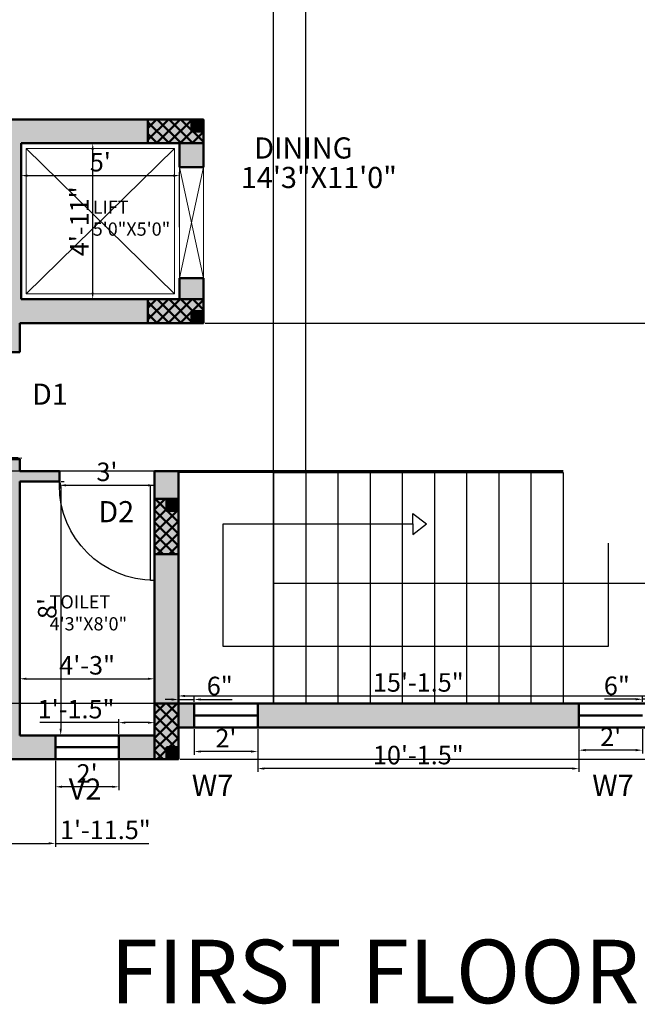
# Model space of a CAD drawing. Units: inches. Extents: x 1749 to 3550, y 1117 to 2383.
# Tile 2 of 15: x 2044 to 2277, y 1117 to 1490. Entities that reach past the tile are written whole.
import ezdxf

# ---------------------------------------------------------------- set-up
doc = ezdxf.new("R2010")
doc.units = ezdxf.units.IN
for name, color, linetype, lineweight in [('A-ANNO-DIMS', 2, 'Continuous', 18), ('A-ANNO-TEXT', 3, 'Continuous', 18), ('A-AREA-IDEN', 7, 'Continuous', 18), ('A-COLS', 10, 'Continuous', 50), ('A-DOOR', 30, 'Continuous', 25), ('A-EQPM', 8, 'Continuous', 18), ('A-FLOR-STRS', 53, 'Continuous', 25), ('A-WALL', 7, 'Continuous', 50), ('A-WALL-PATT', 8, 'Continuous', 13)]:
    doc.layers.add(name, color=color, linetype=linetype, lineweight=lineweight)
doc.styles.get("Standard").update_dxf_attribs({"font": 'arial.ttf'})
doc.dimstyles.new('ISO-25', dxfattribs={"dimtxt": 7, "dimasz": 2.5, "dimexe": 1.25, "dimexo": 0.625, "dimtad": 1, "dimdec": 1, "dimlunit": 3, "dimtxsty": 'Standard', "dimcen": 2.5, "dimadec": 0, "dimazin": 0, "dimtfac": 1, "dimtdec": 1, "dimtmove": 0, "dimatfit": 3, "dimfxl": 1, "dimarcsym": 0})

# ---------------------------------------------------------------- blocks, each defined once
blk = doc.blocks.new('*U12')
for p, q in [((0, 0), (0, 6)), ((40, 0), (40, 6))]:
    blk.add_line(p, q)
blk.add_lwpolyline([(0, 0), (0, -40), (1.75, -40), (1.75, 0)], close=True)
blk.add_arc((0, 0), 40, 270, 0)
blk = doc.blocks.new('*D19')
at = {"layer": 'A-ANNO-DIMS', "color": 0, "lineweight": -2, "ltscale": 0.5, "transparency": 16777216}
for p, q in [((2044.73, 1443.24), (2072.46, 1443.24)), ((2071.21, 1386.74), (2071.21, 1440.74)), ((2044.73, 1384.24), (2072.46, 1384.24))]:
    blk.add_line(p, q, dxfattribs=at)
at = {"layer": 'A-ANNO-DIMS', "color": 0, "ltscale": 0.5, "transparency": 16777216}
for points in [[(2070.8, 1440.74), (2071.63, 1440.74), (2071.21, 1443.24)], [(2070.8, 1386.74), (2071.63, 1386.74), (2071.21, 1384.24)]]:
    blk.add_solid(points, dxfattribs=at)
at = {"layer": 'Defpoints', "color": 0, "ltscale": 0.5, "transparency": 16777216}
for p in [(2044.1, 1443.24), (2071.21, 1443.24), (2044.1, 1384.24)]:
    blk.add_point(p, dxfattribs=at)
at = {"layer": 'A-ANNO-DIMS', "color": 0, "ltscale": 0.5, "transparency": 16777216, "insert": (2067.08, 1413.74), "char_height": 7, "attachment_point": 5, "rotation": 90}
blk.add_mtext('4\'-11"', dxfattribs=at)
blk = doc.blocks.new('*D20')
at = {"layer": 'A-ANNO-DIMS', "color": 0, "lineweight": -2, "ltscale": 0.5, "transparency": 16777216}
for p, q in [((2044.1, 1411.57), (2044.1, 1432.28)), ((2046.6, 1431.03), (2101.6, 1431.03)), ((2104.1, 1411.57), (2104.1, 1432.28))]:
    blk.add_line(p, q, dxfattribs=at)
at = {"layer": 'A-ANNO-DIMS', "color": 0, "ltscale": 0.5, "transparency": 16777216}
for points in [[(2046.6, 1431.44), (2046.6, 1430.61), (2044.1, 1431.03)], [(2101.6, 1431.44), (2101.6, 1430.61), (2104.1, 1431.03)]]:
    blk.add_solid(points, dxfattribs=at)
at = {"layer": 'Defpoints', "color": 0, "ltscale": 0.5, "transparency": 16777216}
for p in [(2104.1, 1431.03), (2044.1, 1410.95), (2104.1, 1410.95)]:
    blk.add_point(p, dxfattribs=at)
at = {"layer": 'A-ANNO-DIMS', "color": 0, "ltscale": 0.5, "transparency": 16777216, "insert": (2074.1, 1435.21), "char_height": 7, "attachment_point": 5}
blk.add_mtext("5'", dxfattribs=at)
blk = doc.blocks.new('*D25')
at = {"layer": 'A-ANNO-DIMS', "color": 0, "lineweight": -2, "ltscale": 0.5, "transparency": 16777216}
for p, q in [((2043.6, 1219.87), (2043.6, 1241.89)), ((2046.1, 1240.64), (2092.1, 1240.64)), ((2094.6, 1219.87), (2094.6, 1241.89))]:
    blk.add_line(p, q, dxfattribs=at)
at = {"layer": 'A-ANNO-DIMS', "color": 0, "ltscale": 0.5, "transparency": 16777216}
for points in [[(2046.1, 1241.06), (2046.1, 1240.22), (2043.6, 1240.64)], [(2092.1, 1241.06), (2092.1, 1240.22), (2094.6, 1240.64)]]:
    blk.add_solid(points, dxfattribs=at)
at = {"layer": 'Defpoints', "color": 0, "ltscale": 0.5, "transparency": 16777216}
for p in [(2094.6, 1240.64), (2043.6, 1219.24), (2094.6, 1219.24)]:
    blk.add_point(p, dxfattribs=at)
at = {"layer": 'A-ANNO-DIMS', "color": 0, "ltscale": 0.5, "transparency": 16777216, "insert": (2069.1, 1244.84), "char_height": 7, "attachment_point": 5}
blk.add_mtext('4\'-3"', dxfattribs=at)
blk = doc.blocks.new('*D26')
at = {"layer": 'A-ANNO-DIMS', "color": 0, "lineweight": -2, "ltscale": 0.5, "transparency": 16777216}
for p, q in [((2059.23, 1315.24), (2060.36, 1315.24)), ((2059.11, 1312.74), (2059.11, 1221.74)), ((2059.23, 1219.24), (2060.36, 1219.24))]:
    blk.add_line(p, q, dxfattribs=at)
at = {"layer": 'A-ANNO-DIMS', "color": 0, "ltscale": 0.5, "transparency": 16777216}
for points in [[(2058.69, 1312.74), (2059.53, 1312.74), (2059.11, 1315.24)], [(2058.69, 1221.74), (2059.53, 1221.74), (2059.11, 1219.24)]]:
    blk.add_solid(points, dxfattribs=at)
at = {"layer": 'Defpoints', "color": 0, "ltscale": 0.5, "transparency": 16777216}
for p in [(2058.6, 1315.24), (2058.6, 1219.24), (2059.11, 1219.24)]:
    blk.add_point(p, dxfattribs=at)
at = {"layer": 'A-ANNO-DIMS', "color": 0, "ltscale": 0.5, "transparency": 16777216, "insert": (2054.91, 1267.24), "char_height": 7, "attachment_point": 5, "rotation": 90}
blk.add_mtext("8'", dxfattribs=at)
blk = doc.blocks.new('*D54')
at = {"layer": 'A-ANNO-DIMS', "color": 0, "lineweight": -2, "ltscale": 0.5, "transparency": 16777216}
for p, q in [((2279.1, 1231.87), (2279.1, 1234.15)), ((2285.1, 1231.87), (2285.1, 1234.15)), ((2276.6, 1232.9), (2264.77, 1232.9)), ((2285.1, 1232.9), (2279.1, 1232.9)), ((2287.6, 1232.9), (2290.1, 1232.9))]:
    blk.add_line(p, q, dxfattribs=at)
at = {"layer": 'A-ANNO-DIMS', "color": 0, "ltscale": 0.5, "transparency": 16777216}
for points in [[(2276.6, 1233.32), (2276.6, 1232.49), (2279.1, 1232.9)], [(2287.6, 1233.32), (2287.6, 1232.49), (2285.1, 1232.9)]]:
    blk.add_solid(points, dxfattribs=at)
at = {"layer": 'Defpoints', "color": 0, "ltscale": 0.5, "transparency": 16777216}
for p in [(2279.1, 1232.9), (2279.1, 1231.24), (2285.1, 1231.24)]:
    blk.add_point(p, dxfattribs=at)
at = {"layer": 'A-ANNO-DIMS', "color": 0, "ltscale": 0.5, "transparency": 16777216, "insert": (2269.44, 1237.1), "char_height": 7, "attachment_point": 5}
blk.add_mtext('6"', dxfattribs=at)
blk = doc.blocks.new('*D55')
at = {"layer": 'A-ANNO-DIMS', "color": 0, "lineweight": -2, "ltscale": 0.5, "transparency": 16777216}
for p, q in [((2255.1, 1221.62), (2255.1, 1212.39)), ((2279.1, 1221.62), (2279.1, 1212.39)), ((2276.6, 1213.64), (2257.6, 1213.64))]:
    blk.add_line(p, q, dxfattribs=at)
at = {"layer": 'A-ANNO-DIMS', "color": 0, "ltscale": 0.5, "transparency": 16777216}
for points in [[(2257.6, 1214.06), (2257.6, 1213.23), (2255.1, 1213.64)], [(2276.6, 1214.06), (2276.6, 1213.23), (2279.1, 1213.64)]]:
    blk.add_solid(points, dxfattribs=at)
at = {"layer": 'Defpoints', "color": 0, "ltscale": 0.5, "transparency": 16777216}
for p in [(2255.1, 1222.24), (2279.1, 1222.24), (2255.1, 1213.64)]:
    blk.add_point(p, dxfattribs=at)
at = {"layer": 'A-ANNO-DIMS', "color": 0, "ltscale": 0.5, "transparency": 16777216, "insert": (2267.1, 1217.78), "char_height": 7, "attachment_point": 5}
blk.add_mtext("2'", dxfattribs=at)
blk = doc.blocks.new('*D56')
at = {"layer": 'A-ANNO-DIMS', "color": 0, "lineweight": -2, "ltscale": 0.5, "transparency": 16777216}
for p, q in [((2133.6, 1221.62), (2133.6, 1205.42)), ((2255.1, 1221.62), (2255.1, 1205.42)), ((2252.6, 1206.67), (2136.1, 1206.67))]:
    blk.add_line(p, q, dxfattribs=at)
at = {"layer": 'A-ANNO-DIMS', "color": 0, "ltscale": 0.5, "transparency": 16777216}
for points in [[(2136.1, 1207.09), (2136.1, 1206.26), (2133.6, 1206.67)], [(2252.6, 1207.09), (2252.6, 1206.26), (2255.1, 1206.67)]]:
    blk.add_solid(points, dxfattribs=at)
at = {"layer": 'Defpoints', "color": 0, "ltscale": 0.5, "transparency": 16777216}
for p in [(2133.6, 1222.24), (2255.1, 1222.24), (2133.6, 1206.67)]:
    blk.add_point(p, dxfattribs=at)
at = {"layer": 'A-ANNO-DIMS', "color": 0, "ltscale": 0.5, "transparency": 16777216, "insert": (2194.35, 1210.87), "char_height": 7, "attachment_point": 5}
blk.add_mtext('10\'-1.5"', dxfattribs=at)
blk = doc.blocks.new('*D57')
at = {"layer": 'A-ANNO-DIMS', "color": 0, "lineweight": -2, "ltscale": 0.5, "transparency": 16777216}
for p, q in [((2109.6, 1221.62), (2109.6, 1211.87)), ((2133.6, 1221.62), (2133.6, 1211.87)), ((2131.1, 1213.12), (2112.1, 1213.12))]:
    blk.add_line(p, q, dxfattribs=at)
at = {"layer": 'A-ANNO-DIMS', "color": 0, "ltscale": 0.5, "transparency": 16777216}
for points in [[(2112.1, 1213.54), (2112.1, 1212.71), (2109.6, 1213.12)], [(2131.1, 1213.54), (2131.1, 1212.71), (2133.6, 1213.12)]]:
    blk.add_solid(points, dxfattribs=at)
at = {"layer": 'Defpoints', "color": 0, "ltscale": 0.5, "transparency": 16777216}
for p in [(2109.6, 1222.24), (2133.6, 1222.24), (2109.6, 1213.12)]:
    blk.add_point(p, dxfattribs=at)
at = {"layer": 'A-ANNO-DIMS', "color": 0, "ltscale": 0.5, "transparency": 16777216, "insert": (2121.6, 1217.26), "char_height": 7, "attachment_point": 5}
blk.add_mtext("2'", dxfattribs=at)
blk = doc.blocks.new('*D58')
at = {"layer": 'A-ANNO-DIMS', "color": 0, "lineweight": -2, "ltscale": 0.5, "transparency": 16777216}
for p, q in [((2103.6, 1231.87), (2103.6, 1234.06)), ((2109.6, 1231.87), (2109.6, 1234.06)), ((2101.1, 1232.81), (2098.6, 1232.81)), ((2103.6, 1232.81), (2109.6, 1232.81)), ((2112.1, 1232.81), (2123.94, 1232.81))]:
    blk.add_line(p, q, dxfattribs=at)
at = {"layer": 'A-ANNO-DIMS', "color": 0, "ltscale": 0.5, "transparency": 16777216}
for points in [[(2101.1, 1233.23), (2101.1, 1232.4), (2103.6, 1232.81)], [(2112.1, 1233.23), (2112.1, 1232.4), (2109.6, 1232.81)]]:
    blk.add_solid(points, dxfattribs=at)
at = {"layer": 'Defpoints', "color": 0, "ltscale": 0.5, "transparency": 16777216}
for p in [(2103.6, 1231.24), (2109.6, 1232.81), (2109.6, 1231.24)]:
    blk.add_point(p, dxfattribs=at)
at = {"layer": 'A-ANNO-DIMS', "color": 0, "ltscale": 0.5, "transparency": 16777216, "insert": (2119.27, 1237.01), "char_height": 7, "attachment_point": 5}
blk.add_mtext('6"', dxfattribs=at)
blk = doc.blocks.new('*D59')
at = {"layer": 'A-ANNO-DIMS', "color": 0, "lineweight": -2, "ltscale": 0.5, "transparency": 16777216}
for p, q in [((2081.1, 1224.06), (2051.25, 1224.06)), ((2081.1, 1219.87), (2081.1, 1225.31)), ((2092.1, 1224.06), (2083.6, 1224.06)), ((2094.6, 1219.87), (2094.6, 1225.31))]:
    blk.add_line(p, q, dxfattribs=at)
at = {"layer": 'A-ANNO-DIMS', "color": 0, "ltscale": 0.5, "transparency": 16777216}
for points in [[(2083.6, 1224.47), (2083.6, 1223.64), (2081.1, 1224.06)], [(2092.1, 1224.47), (2092.1, 1223.64), (2094.6, 1224.06)]]:
    blk.add_solid(points, dxfattribs=at)
at = {"layer": 'Defpoints', "color": 0, "ltscale": 0.5, "transparency": 16777216}
for p in [(2081.1, 1224.06), (2081.1, 1219.24), (2094.6, 1219.24)]:
    blk.add_point(p, dxfattribs=at)
at = {"layer": 'A-ANNO-DIMS', "color": 0, "ltscale": 0.5, "transparency": 16777216, "insert": (2064.93, 1228.26), "char_height": 7, "attachment_point": 5}
blk.add_mtext('1\'-1.5"', dxfattribs=at)
blk = doc.blocks.new('*D60')
at = {"layer": 'A-ANNO-DIMS', "color": 0, "lineweight": -2, "ltscale": 0.5, "transparency": 16777216}
for p, q in [((2057.1, 1209.62), (2057.1, 1198.53)), ((2081.1, 1209.62), (2081.1, 1198.53)), ((2078.6, 1199.78), (2059.6, 1199.78))]:
    blk.add_line(p, q, dxfattribs=at)
at = {"layer": 'A-ANNO-DIMS', "color": 0, "ltscale": 0.5, "transparency": 16777216}
for points in [[(2059.6, 1200.2), (2059.6, 1199.36), (2057.1, 1199.78)], [(2078.6, 1200.2), (2078.6, 1199.36), (2081.1, 1199.78)]]:
    blk.add_solid(points, dxfattribs=at)
at = {"layer": 'Defpoints', "color": 0, "ltscale": 0.5, "transparency": 16777216}
for p in [(2057.1, 1210.24), (2081.1, 1210.24), (2057.1, 1199.78)]:
    blk.add_point(p, dxfattribs=at)
at = {"layer": 'A-ANNO-DIMS', "color": 0, "ltscale": 0.5, "transparency": 16777216, "insert": (2069.1, 1203.92), "char_height": 7, "attachment_point": 5}
blk.add_mtext("2'", dxfattribs=at)
blk = doc.blocks.new('*D61')
at = {"layer": 'A-ANNO-DIMS', "color": 0, "lineweight": -2, "ltscale": 0.5, "transparency": 16777216}
for p, q in [((2033.6, 1209.62), (2033.6, 1177.12)), ((2057.1, 1209.62), (2057.1, 1177.12)), ((2036.1, 1178.37), (2054.6, 1178.37)), ((2057.1, 1178.37), (2092.4, 1178.37))]:
    blk.add_line(p, q, dxfattribs=at)
at = {"layer": 'A-ANNO-DIMS', "color": 0, "ltscale": 0.5, "transparency": 16777216}
for points in [[(2036.1, 1178.79), (2036.1, 1177.95), (2033.6, 1178.37)], [(2054.6, 1178.79), (2054.6, 1177.95), (2057.1, 1178.37)]]:
    blk.add_solid(points, dxfattribs=at)
at = {"layer": 'Defpoints', "color": 0, "ltscale": 0.5, "transparency": 16777216}
for p in [(2033.6, 1210.24), (2057.1, 1210.24), (2057.1, 1178.37)]:
    blk.add_point(p, dxfattribs=at)
at = {"layer": 'A-ANNO-DIMS', "color": 0, "ltscale": 0.5, "transparency": 16777216, "insert": (2076, 1182.57), "char_height": 7, "attachment_point": 5}
blk.add_mtext('1\'-11.5"', dxfattribs=at)
blk = doc.blocks.new('*D97')
at = {"layer": 'A-ANNO-DIMS', "color": 0, "lineweight": -2, "ltscale": 0.5, "transparency": 16777216}
for p, q in [((2042.16, 1364.23), (2038.93, 1364.23)), ((2040.18, 1326.73), (2040.18, 1361.73)), ((2042.98, 1324.23), (2038.93, 1324.23))]:
    blk.add_line(p, q, dxfattribs=at)
at = {"layer": 'A-ANNO-DIMS', "color": 0, "ltscale": 0.5, "transparency": 16777216}
for points in [[(2039.77, 1361.73), (2040.6, 1361.73), (2040.18, 1364.23)], [(2039.77, 1326.73), (2040.6, 1326.73), (2040.18, 1324.23)]]:
    blk.add_solid(points, dxfattribs=at)
at = {"layer": 'Defpoints', "color": 0, "ltscale": 0.5, "transparency": 16777216}
for p in [(2040.18, 1364.23), (2042.78, 1364.23), (2043.6, 1324.23)]:
    blk.add_point(p, dxfattribs=at)
at = {"layer": 'A-ANNO-DIMS', "color": 0, "ltscale": 0.5, "transparency": 16777216, "insert": (2035.98, 1344.23), "char_height": 7, "attachment_point": 5, "rotation": 90}
blk.add_mtext('3\'-4"', dxfattribs=at)
blk = doc.blocks.new('*D98')
at = {"layer": 'A-ANNO-DIMS', "color": 0, "lineweight": -2, "ltscale": 0.5, "transparency": 16777216}
for p, q in [((2058.6, 1318.62), (2058.6, 1312.59)), ((2094.6, 1318.62), (2094.6, 1312.59)), ((2061.1, 1313.84), (2092.1, 1313.84))]:
    blk.add_line(p, q, dxfattribs=at)
at = {"layer": 'A-ANNO-DIMS', "color": 0, "ltscale": 0.5, "transparency": 16777216}
for points in [[(2061.1, 1314.26), (2061.1, 1313.43), (2058.6, 1313.84)], [(2092.1, 1314.26), (2092.1, 1313.43), (2094.6, 1313.84)]]:
    blk.add_solid(points, dxfattribs=at)
at = {"layer": 'Defpoints', "color": 0, "ltscale": 0.5, "transparency": 16777216}
for p in [(2058.6, 1319.24), (2094.6, 1319.24), (2094.6, 1313.84)]:
    blk.add_point(p, dxfattribs=at)
at = {"layer": 'A-ANNO-DIMS', "color": 0, "ltscale": 0.5, "transparency": 16777216, "insert": (2076.6, 1318.04), "char_height": 7, "attachment_point": 5}
blk.add_mtext("3'", dxfattribs=at)
blk = doc.blocks.new('*D150')
at = {"layer": 'A-ANNO-DIMS', "color": 0, "lineweight": -2, "ltscale": 0.5, "transparency": 16777216}
for p, q in [((2103.6, 1231.87), (2103.6, 1235.4)), ((2106.1, 1234.15), (2282.6, 1234.15)), ((2285.1, 1231.87), (2285.1, 1235.4))]:
    blk.add_line(p, q, dxfattribs=at)
at = {"layer": 'A-ANNO-DIMS', "color": 0, "ltscale": 0.5, "transparency": 16777216}
for points in [[(2106.1, 1234.57), (2106.1, 1233.74), (2103.6, 1234.15)], [(2282.6, 1234.57), (2282.6, 1233.74), (2285.1, 1234.15)]]:
    blk.add_solid(points, dxfattribs=at)
at = {"layer": 'Defpoints', "color": 0, "ltscale": 0.5, "transparency": 16777216}
for p in [(2285.1, 1234.15), (2103.6, 1231.24), (2285.1, 1231.24)]:
    blk.add_point(p, dxfattribs=at)
at = {"layer": 'A-ANNO-DIMS', "color": 0, "ltscale": 0.5, "transparency": 16777216, "insert": (2194.35, 1238.35), "char_height": 7, "attachment_point": 5}
blk.add_mtext('15\'-1.5"', dxfattribs=at)
blk = doc.blocks.new('LIFT-B')
at = {"ltscale": 0.5}
for p, q in [((0, 55), (56, 55)), ((0, 0), (0, 55)), ((56, 55), (0, 0)), ((0, 55), (56, 0)), ((56, 55), (56, 0)), ((56, 0), (0, 0))]:
    blk.add_line(p, q, dxfattribs=at)
blk = doc.blocks.new('*D176')
at = {"layer": 'A-ANNO-DIMS', "color": 0, "lineweight": -2, "ltscale": 0.5, "transparency": 16777216}
for p, q in [((2102.98, 1319.24), (1818.35, 1319.24)), ((1819.6, 1233.74), (1819.6, 1316.74)), ((2102.98, 1231.24), (1818.35, 1231.24))]:
    blk.add_line(p, q, dxfattribs=at)
at = {"layer": 'A-ANNO-DIMS', "color": 0, "ltscale": 0.5, "transparency": 16777216}
for points in [[(1819.19, 1316.74), (1820.02, 1316.74), (1819.6, 1319.24)], [(1819.19, 1233.74), (1820.02, 1233.74), (1819.6, 1231.24)]]:
    blk.add_solid(points, dxfattribs=at)
at = {"layer": 'Defpoints', "color": 0, "ltscale": 0.5, "transparency": 16777216}
for p in [(1819.6, 1319.24), (2103.6, 1319.24), (2103.6, 1231.24)]:
    blk.add_point(p, dxfattribs=at)
at = {"layer": 'A-ANNO-DIMS', "color": 0, "ltscale": 0.5, "transparency": 16777216, "insert": (1815.48, 1275.24), "char_height": 7, "attachment_point": 5, "rotation": 90}
blk.add_mtext('7\'-4"', dxfattribs=at)
blk = doc.blocks.new('*D177')
at = {"layer": 'A-ANNO-DIMS', "color": 0, "lineweight": -2, "ltscale": 0.5, "transparency": 16777216}
for p, q in [((2139.6, 1319.37), (2139.6, 1679.49)), ((2142.1, 1678.24), (2149.27, 1678.24)), ((2151.77, 1319.37), (2151.77, 1679.49)), ((2151.77, 1678.24), (2173.47, 1678.24))]:
    blk.add_line(p, q, dxfattribs=at)
at = {"layer": 'A-ANNO-DIMS', "color": 0, "ltscale": 0.5, "transparency": 16777216}
for points in [[(2142.1, 1678.66), (2142.1, 1677.83), (2139.6, 1678.24)], [(2149.27, 1678.66), (2149.27, 1677.83), (2151.77, 1678.24)]]:
    blk.add_solid(points, dxfattribs=at)
at = {"layer": 'Defpoints', "color": 0, "ltscale": 0.5, "transparency": 16777216}
for p in [(2151.77, 1678.24), (2139.6, 1318.74), (2151.77, 1318.74)]:
    blk.add_point(p, dxfattribs=at)
at = {"layer": 'A-ANNO-DIMS', "color": 0, "ltscale": 0.5, "transparency": 16777216, "insert": (2163.87, 1682.44), "char_height": 7, "attachment_point": 5}
blk.add_mtext('1\'-0"', dxfattribs=at)
blk = doc.blocks.new('*D179')
at = {"layer": 'A-ANNO-DIMS', "color": 0, "lineweight": -2, "ltscale": 0.5, "transparency": 16777216}
for p, q in [((2113.73, 1375.24), (2559.85, 1375.24)), ((2558.6, 1212.74), (2558.6, 1372.74)), ((2104.23, 1210.24), (2559.85, 1210.24))]:
    blk.add_line(p, q, dxfattribs=at)
at = {"layer": 'A-ANNO-DIMS', "color": 0, "ltscale": 0.5, "transparency": 16777216}
for points in [[(2558.19, 1372.74), (2559.02, 1372.74), (2558.6, 1375.24)], [(2558.19, 1212.74), (2559.02, 1212.74), (2558.6, 1210.24)]]:
    blk.add_solid(points, dxfattribs=at)
at = {"layer": 'Defpoints', "color": 0, "ltscale": 0.5, "transparency": 16777216}
for p in [(2113.1, 1375.24), (2558.6, 1375.24), (2103.6, 1210.24)]:
    blk.add_point(p, dxfattribs=at)
at = {"layer": 'A-ANNO-DIMS', "color": 0, "ltscale": 0.5, "transparency": 16777216, "insert": (2554.4, 1292.74), "char_height": 7, "attachment_point": 5, "rotation": 90}
blk.add_mtext('13\'-9"', dxfattribs=at)

msp = doc.modelspace()

# ---------------------------------------------------------------- hatches: boundary and pattern name
at = {"layer": 'A-COLS', "ltscale": 10}
h = msp.add_hatch(dxfattribs=at)
h.set_pattern_fill('ANSI37', color=256)
h.set_pattern_definition([(45, (440.86, 85.1368), (-2.245064, 2.245064), []), (135, (440.86, 85.1368), (-2.245064, -2.245064), [])])
h.paths.add_polyline_path([(2113.1, 1443.24), (2113.1, 1452.24), (2092.1, 1452.24), (2092.1, 1443.24)])
h = msp.add_hatch(color=256, dxfattribs=at)
h.dxf.hatch_style = 1
h.paths.add_polyline_path([(2108.6, 1452.24), (2108.6, 1447.74), (2113.1, 1447.74), (2113.1, 1452.24)])
h = msp.add_hatch(dxfattribs=at)
h.set_pattern_fill('ANSI37', color=256)
h.set_pattern_definition([(45, (440.86, 17.1368), (-2.245064, 2.245064), []), (135, (440.86, 17.1368), (-2.245064, -2.245064), [])])
h.paths.add_polyline_path([(2113.1, 1375.24), (2113.1, 1384.24), (2092.1, 1384.24), (2092.1, 1375.24)])
h = msp.add_hatch(color=256, dxfattribs=at)
h.dxf.hatch_style = 1
h.paths.add_polyline_path([(2108.6, 1379.74), (2108.6, 1375.24), (2113.1, 1375.24), (2113.1, 1379.74)])
h = msp.add_hatch(dxfattribs=at)
h.set_pattern_fill('ANSI37', color=256, angle=90)
h.set_pattern_definition([(135, (3461.7103, -363.5015), (-2.245064, -2.245064), []), (225, (3461.7103, -363.5015), (2.245064, -2.245064), [])])
h.paths.add_polyline_path([(2103.6, 1308.74), (2094.6, 1308.74), (2094.6, 1287.74), (2103.6, 1287.74)])
h = msp.add_hatch(color=256, dxfattribs=at)
h.dxf.hatch_style = 1
h.paths.add_polyline_path([(2099.1, 1308.74), (2099.1, 1304.24), (2103.6, 1304.24), (2103.6, 1308.74)])
h = msp.add_hatch(dxfattribs=at)
h.set_pattern_fill('ANSI37', color=256, angle=90)
h.set_pattern_definition([(135, (3461.7103, -441.0015), (-2.245064, -2.245064), []), (225, (3461.7103, -441.0015), (2.245064, -2.245064), [])])
h.paths.add_polyline_path([(2103.6, 1231.24), (2094.6, 1231.24), (2094.6, 1210.24), (2103.6, 1210.24)])
h = msp.add_hatch(color=256, dxfattribs=at)
h.dxf.hatch_style = 1
h.paths.add_polyline_path([(2099.1, 1214.74), (2099.1, 1210.24), (2103.6, 1210.24), (2103.6, 1214.74)])
at = {"layer": 'A-WALL-PATT', "ltscale": 10}
h = msp.add_hatch(color=256, dxfattribs=at)
h.dxf.hatch_style = 1
h.paths.add_polyline_path([(1971.1, 1448.24), (1971.1, 1425.74), (1975.1, 1425.74), (1975.1, 1448.24), (2035.1, 1448.24), (2035.1, 1379.24), (2011.1, 1379.24), (2011.1, 1375.24), (2039.6, 1375.24), (2039.6, 1364.24), (2043.6, 1364.24), (2043.6, 1375.24), (2113.1, 1375.24), (2113.1, 1392.24), (2104.1, 1392.24), (2104.1, 1379.24), (2044.1, 1379.24), (2044.1, 1443.24), (2104.1, 1443.24), (2104.1, 1434.24), (2113.1, 1434.24), (2113.1, 1452.24), (2104.1, 1452.24), (1868.6, 1452.24), (1868.6, 1473.24), (1859.6, 1473.24), (1859.6, 1425.74), (1868.6, 1425.74), (1868.6, 1448.24), (1907.6, 1448.24), (1908.1, 1448.24)])
h = msp.add_hatch(color=256, dxfattribs=at)
h.dxf.hatch_style = 1
h.paths.add_polyline_path([(2044.1, 1384.24), (2044.1, 1443.24), (2104.1, 1443.24), (2104.1, 1434.24), (2113.1, 1434.24), (2113.1, 1447.74), (2108.6, 1447.74), (2108.6, 1452.24), (2104.1, 1452.24), (1868.6, 1452.24), (1868.6, 1448.24), (1907.6, 1448.24), (1908.1, 1448.24), (1971.1, 1448.24), (1971.1, 1425.74), (1975.1, 1425.74), (1975.1, 1448.24), (2035.1, 1448.24), (2035.1, 1379.24), (2011.1, 1379.24), (2011.1, 1375.24), (2039.6, 1375.24), (2039.6, 1364.24), (2043.6, 1364.24), (2043.6, 1375.24), (2092.1, 1375.24), (2092.1, 1384.24)])
h.paths.add_polyline_path([(2092.1, 1384.24), (2092.1, 1375.24), (2108.6, 1375.24), (2108.6, 1379.74), (2113.1, 1379.74), (2113.1, 1384.24)], flags=17)
h = msp.add_hatch(color=256, dxfattribs=at)
h.dxf.hatch_style = 1
h.paths.add_polyline_path([(2039.6, 1219.24), (2033.6, 1219.24), (2033.6, 1210.24), (2057.1, 1210.24), (2057.1, 1219.24), (2043.6, 1219.24), (2043.6, 1315.24), (2058.6, 1315.24), (2058.6, 1319.24), (2043.6, 1319.24), (2043.6, 1323.74), (2039.6, 1323.74)])
h = msp.add_hatch(color=256, dxfattribs=at)
h.dxf.hatch_style = 1
h.paths.add_polyline_path([(2103.6, 1319.24), (2094.6, 1319.24), (2094.6, 1315.24), (2094.6, 1219.24), (2081.1, 1219.24), (2081.1, 1210.24), (2103.6, 1210.24), (2103.6, 1222.24), (2109.6, 1222.24), (2109.6, 1231.24), (2103.6, 1231.24)])
h = msp.add_hatch(color=256, dxfattribs=at)
h.dxf.hatch_style = 1
h.paths.add_polyline_path([(2133.6, 1231.24), (2133.6, 1222.24), (2255.1, 1222.24), (2255.1, 1231.24)])

# ---------------------------------------------------------------- linework, layer by layer
at = {"layer": 'A-COLS', "ltscale": 10}
for points in [[(2092.1, 1452.24), (2113.1, 1452.24), (2113.1, 1443.24), (2092.1, 1443.24)], [(2108.6, 1452.24), (2113.1, 1452.24), (2113.1, 1447.74), (2108.6, 1447.74)], [(2092.1, 1384.24), (2113.1, 1384.24), (2113.1, 1375.24), (2092.1, 1375.24)], [(2108.6, 1379.74), (2113.1, 1379.74), (2113.1, 1375.24), (2108.6, 1375.24)], [(2094.6, 1287.74), (2094.6, 1308.74), (2103.6, 1308.74), (2103.6, 1287.74)], [(2099.1, 1308.74), (2103.6, 1308.74), (2103.6, 1304.24), (2099.1, 1304.24)], [(2094.6, 1210.24), (2094.6, 1231.24), (2103.6, 1231.24), (2103.6, 1210.24)], [(2099.1, 1214.74), (2103.6, 1214.74), (2103.6, 1210.24), (2099.1, 1210.24)]]:
    msp.add_lwpolyline(points, close=True, dxfattribs=at)
at = {"layer": 'A-EQPM', "ltscale": 0.5}
for p, q in [((2044.1, 1443.24), (2044.1, 1441.24)), ((2104.1, 1441.24), (2104.1, 1384.24)), ((2113.1, 1434.24), (2104.1, 1434.24)), ((2104.1, 1434.24), (2104.1, 1392.24)), ((2113.1, 1392.24), (2104.1, 1434.24)), ((2104.1, 1434.24), (2113.1, 1434.24)), ((2113.1, 1434.24), (2104.1, 1392.24)), ((2113.1, 1392.24), (2113.1, 1434.24)), ((2104.1, 1392.24), (2113.1, 1392.24)), ((2104.1, 1384.24), (2104.1, 1386.24))]:
    msp.add_line(p, q, dxfattribs=at)
at = {"layer": 'A-FLOR-STRS', "ltscale": 0.5}
for p, q in [((2139.6, 1318.74), (2103.6, 1318.74)), ((2139.6, 1231.24), (2139.6, 1318.74)), ((2139.6, 1318.74), (2249.1, 1318.74)), ((2139.6, 1318.74), (2139.6, 1231.24)), ((2151.77, 1318.74), (2151.77, 1231.24)), ((2163.94, 1318.74), (2163.94, 1231.24)), ((2176.1, 1318.74), (2176.1, 1231.24)), ((2188.27, 1318.74), (2188.27, 1231.24)), ((2200.44, 1318.74), (2200.44, 1231.24)), ((2212.6, 1318.74), (2212.6, 1231.24)), ((2224.77, 1318.74), (2224.77, 1231.24)), ((2236.94, 1318.74), (2236.94, 1231.24)), ((2249.1, 1318.74), (2249.1, 1231.24)), ((2192.27, 1299.22), (2192.27, 1303.16)), ((2192.27, 1303.16), (2197.49, 1299.22)), ((2120.54, 1252.88), (2120.54, 1299.22)), ((2120.54, 1299.22), (2192.27, 1299.22)), ((2192.27, 1299.22), (2192.27, 1295.27)), ((2192.27, 1295.27), (2197.49, 1299.22)), ((2266.19, 1291.97), (2266.19, 1252.88)), ((2285.1, 1276.74), (2139.6, 1276.74)), ((2266.19, 1252.88), (2120.54, 1252.88)), ((2103.6, 1231.24), (2139.6, 1231.24))]:
    msp.add_line(p, q, dxfattribs=at)
at = {"layer": 'A-WALL', "ltscale": 0.2}
for p, q in [((1868.6, 1452.24), (2104.1, 1452.24)), ((2104.1, 1452.24), (2113.1, 1452.24)), ((2113.1, 1452.24), (2113.1, 1434.24)), ((2044.1, 1443.24), (2044.1, 1384.24)), ((2044.1, 1443.24), (2104.1, 1443.24)), ((2104.1, 1443.24), (2104.1, 1434.24)), ((2104.1, 1434.24), (2113.1, 1434.24)), ((2104.1, 1392.24), (2113.1, 1392.24)), ((2104.1, 1392.24), (2104.1, 1384.24)), ((2113.1, 1392.24), (2113.1, 1375.24)), ((2044.1, 1384.24), (2104.1, 1384.24)), ((2043.6, 1375.24), (2043.6, 1364.24)), ((2043.6, 1375.24), (2113.1, 1375.24)), ((2043.6, 1364.24), (2039.6, 1364.24)), ((2043.6, 1323.74), (2039.6, 1323.74)), ((2043.6, 1323.74), (2043.6, 1319.24)), ((2043.6, 1319.24), (2058.6, 1319.24)), ((2058.6, 1315.24), (2058.6, 1319.24)), ((2094.6, 1315.24), (2094.6, 1319.24)), ((2094.6, 1319.24), (2103.6, 1319.24)), ((2103.6, 1319.24), (2103.6, 1231.24)), ((2043.6, 1315.24), (2058.6, 1315.24)), ((2043.6, 1315.24), (2043.6, 1219.24)), ((2094.6, 1315.24), (2094.6, 1219.24)), ((2103.6, 1231.24), (2285.1, 1231.24)), ((2109.6, 1231.24), (2109.6, 1222.24)), ((2133.6, 1231.24), (2133.6, 1222.24)), ((2255.1, 1231.24), (2255.1, 1222.24)), ((2109.6, 1226.74), (2133.6, 1226.74)), ((2255.1, 1226.74), (2279.1, 1226.74)), ((2103.6, 1219.24), (2103.6, 1222.24)), ((2103.6, 1222.24), (2285.1, 1222.24)), ((2103.6, 1222.24), (2103.6, 1210.24)), ((2043.6, 1219.24), (2094.6, 1219.24)), ((2057.1, 1219.24), (2057.1, 1210.24)), ((2081.1, 1219.24), (2081.1, 1210.24)), ((2057.1, 1214.74), (2081.1, 1214.74)), ((1859.6, 1210.24), (2103.6, 1210.24))]:
    msp.add_line(p, q, dxfattribs=at)
at = {"layer": 'A-WALL', "ltscale": 0.5}
for p, q in [((2103.6, 1319.24), (2249.1, 1319.24)), ((2255.1, 1231.24), (2249.1, 1231.24))]:
    msp.add_line(p, q, dxfattribs=at)

# ---------------------------------------------------------------- block references
at = {"layer": 'A-DOOR', "rotation": 271.1803398379497}
msp.add_blockref('*U12', (2037.61, 1364.12), dxfattribs=at)
at = {"layer": 'A-DOOR', "xscale": -0.9, "yscale": 0.9, "zscale": 0.9}
msp.add_blockref('*U12', (2094.6, 1313.84), dxfattribs=at)
at = {"layer": 'A-EQPM'}
msp.add_blockref('LIFT-B', (2046.1, 1386.24), dxfattribs=at)

# ---------------------------------------------------------------- texts
at = {"layer": 'A-ANNO-TEXT', "ltscale": 0.5}
for s, height, p in [('D1', 8, (2048.25, 1344.33)), ('D2', 8, (2073.33, 1299.87)), ('W7', 8, (2108.71, 1196.33)), ('W7', 8, (2260.15, 1196.33)), ('V2', 8, (2062.17, 1194.92)), ('FIRST FLOOR', 24, (2077.82, 1117.91))]:
    msp.add_text(s, height=height, dxfattribs=at).set_placement(p)
at = {"layer": 'A-AREA-IDEN', "ltscale": 0.5}
msp.add_text('DINING', height=8, rotation=0.0333, dxfattribs=at).set_placement((2132.28, 1437.46))
for s, height, p in [('14\'3"X11\'0"', 8, (2127.24, 1426.31)), ('LIFT', 5, (2071.21, 1416.58)), ('5\'0"X5\'0"', 5, (2071.21, 1408.28)), ('TOILET', 5, (2054.91, 1267.24)), ('4\'3"X8\'0"', 5, (2054.91, 1258.94))]:
    msp.add_text(s, height=height, dxfattribs=at).set_placement(p)

# ---------------------------------------------------------------- dimensions: what is measured, and where the dimension line sits
at = {"layer": 'A-ANNO-DIMS', "ltscale": 0.5}
for base, p1, p2, override, picture, middle in [((2151.77, 1678.24), (2139.6, 1318.74), (2151.77, 1318.74), {"dimdec": 1, "dimlfac": 1, "dimrnd": 0, "dimzin": 1, "dimdsep": 46, "dimlunit": 4, "dimfrac": 2}, '*D177', (2163.87, 1682.44)), ((2104.1, 1431.03), (2044.1, 1410.95), (2104.1, 1410.95), {"dimclrd": 0, "dimclre": 0, "dimclrt": 0}, '*D20', (2074.1, 1435.21)), ((2094.6, 1313.84), (2058.6, 1319.24), (2094.6, 1319.24), {"dimclrd": 0, "dimclre": 0, "dimclrt": 0}, '*D98', (2076.6, 1318.04)), ((2094.6, 1240.64), (2043.6, 1219.24), (2094.6, 1219.24), {"dimclrd": 0, "dimclre": 0, "dimclrt": 0}, '*D25', (2069.1, 1244.84)), ((2109.6, 1232.81), (2103.6, 1231.24), (2109.6, 1231.24), {"dimclrd": 0, "dimclre": 0, "dimclrt": 0}, '*D58', (2119.27, 1237.01)), ((2285.1, 1234.15), (2103.6, 1231.24), (2285.1, 1231.24), {"dimclrd": 0, "dimclre": 0, "dimclrt": 0}, '*D150', (2194.35, 1238.35)), ((2279.1, 1232.9), (2285.1, 1231.24), (2279.1, 1231.24), {"dimclrd": 0, "dimclre": 0, "dimclrt": 0}, '*D54', (2269.44, 1237.1)), ((2081.1, 1224.06), (2094.6, 1219.24), (2081.1, 1219.24), {"dimclrd": 0, "dimclre": 0, "dimclrt": 0}, '*D59', (2064.93, 1228.26)), ((2109.6, 1213.12), (2133.6, 1222.24), (2109.6, 1222.24), {"dimclrd": 0, "dimclre": 0, "dimclrt": 0}, '*D57', (2121.6, 1217.26)), ((2133.6, 1206.67), (2255.1, 1222.24), (2133.6, 1222.24), {"dimclrd": 0, "dimclre": 0, "dimclrt": 0}, '*D56', (2194.35, 1210.87)), ((2255.1, 1213.64), (2279.1, 1222.24), (2255.1, 1222.24), {"dimclrd": 0, "dimclre": 0, "dimclrt": 0}, '*D55', (2267.1, 1217.78)), ((2057.1, 1178.37), (2033.6, 1210.24), (2057.1, 1210.24), {"dimclrd": 0, "dimclre": 0, "dimclrt": 0}, '*D61', (2076, 1182.57)), ((2057.1, 1199.78), (2081.1, 1210.24), (2057.1, 1210.24), {"dimclrd": 0, "dimclre": 0, "dimclrt": 0}, '*D60', (2069.1, 1203.92))]:
    dim = msp.add_linear_dim(base=base, p1=p1, p2=p2, dimstyle='ISO-25', override=override, dxfattribs=at)
    dim.commit()
    dim.dimension.update_dxf_attribs({"geometry": picture, "text_midpoint": middle})
for base, p1, p2, override, picture, middle in [((2071.21, 1443.24), (2044.1, 1384.24), (2044.1, 1443.24), {"dimclrd": 0, "dimclre": 0, "dimclrt": 0}, '*D19', (2067.08, 1413.74)), ((2558.6, 1375.24), (2103.6, 1210.24), (2113.1, 1375.24), {"dimdec": 1, "dimlfac": 1, "dimrnd": 0, "dimzin": 1, "dimdsep": 46, "dimlunit": 4, "dimfrac": 2}, '*D179', (2554.4, 1292.74)), ((2040.18, 1364.23), (2043.6, 1324.23), (2042.78, 1364.23), {"dimclrd": 0, "dimclre": 0, "dimclrt": 0}, '*D97', (2035.98, 1344.23)), ((1819.6, 1319.24), (2103.6, 1231.24), (2103.6, 1319.24), {"dimdec": 1, "dimlfac": 1, "dimrnd": 0, "dimzin": 1, "dimdsep": 46, "dimlunit": 4, "dimfrac": 2}, '*D176', (1815.48, 1275.24)), ((2059.11, 1219.24), (2058.6, 1315.24), (2058.6, 1219.24), {"dimclrd": 0, "dimclre": 0, "dimclrt": 0}, '*D26', (2054.91, 1267.24))]:
    dim = msp.add_linear_dim(base=base, p1=p1, p2=p2, angle=90, dimstyle='ISO-25', override=override, dxfattribs=at)
    dim.commit()
    dim.dimension.update_dxf_attribs({"geometry": picture, "text_midpoint": middle})

doc.saveas('drawing.dxf')
